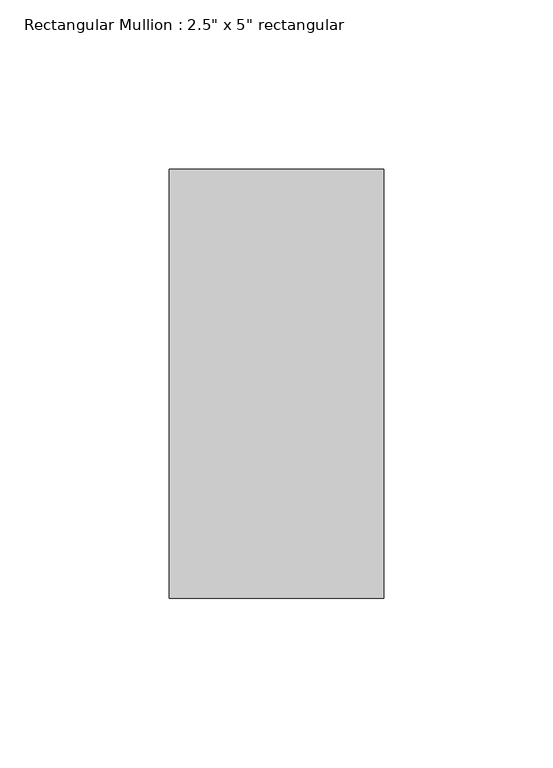
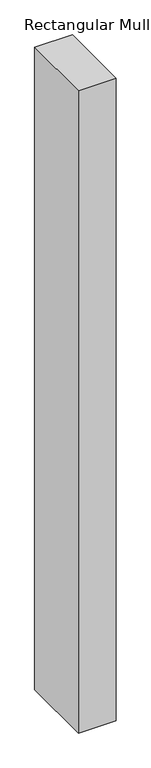
"""IFC4 building model written with IfcOpenShell, lengths in millimetres: member geometry."""

from ifc_helpers import new_model, si_unit, frame, origin, place, context, project, spatial, polyline, outline, extrude, source, transform, mapped, element, save


def member_c1b635f4(model_context):
    return source(origin(), model_context, "Body", "SweptSolid", [
        extrude(outline(polyline([(0.0, 63.5), (0.0, -63.5), (-63.5, -63.5), (-63.5, 63.5), (0.0, 63.5)])), frame((0.0, 0.0, -1142.3491558), z_axis=(0.0, 0.0, 1.0), x_axis=(1.0, 0.0, 0.0)), (0.0, 0.0, 1.0), 1142.3491558),
    ])


if __name__ == "__main__":
    model = new_model("IFC4")
    model_context = context("Model", 3, world=origin())
    ifc_project = project(units=[si_unit("LENGTHUNIT", "METRE", prefix="MILLI")], contexts=[model_context])
    site = spatial("IfcSite", under=ifc_project)
    building = spatial("IfcBuilding", under=site)
    placement = place(None, origin())
    member_shape = member_c1b635f4(model_context)
    element("IfcMember", 1, ObjectType="Rectangular Mullion : 2.5\" x 5\" rectangular", at=placement, inside=building, context=model_context, shape_type="MappedRepresentation", body=[
        mapped(member_shape, transform((0.0, 0.0, 0.0), x_axis=(1.0, 0.0, 0.0), y_axis=(0.0, 1.0, 0.0), z_axis=(0.0, 0.0, 1.0))),
    ])
    save(model, "model.ifc")

# Revit data of these elements
# Type "Rectangular Mullion : 2.5\" x 5\" rectangular"
#   built-in parameter 1007304 = 0.416667 (stored number, unit not read)
#   built-in parameter 1007301 = 0.104167 (stored number, unit not read)
#   built-in parameter 1007300 = 0.104167 (stored number, unit not read)
# Element 1 (IfcMember, "Rectangular Mullion : 2.5\" x 5\" rectangular")
#   Materials on its faces: "Aluminum"
# Materials
#   "Aluminum": class "Metal", colour RGB 247 247 247, transparency 0, Description = "Aluminum 6061", Cost = 0
